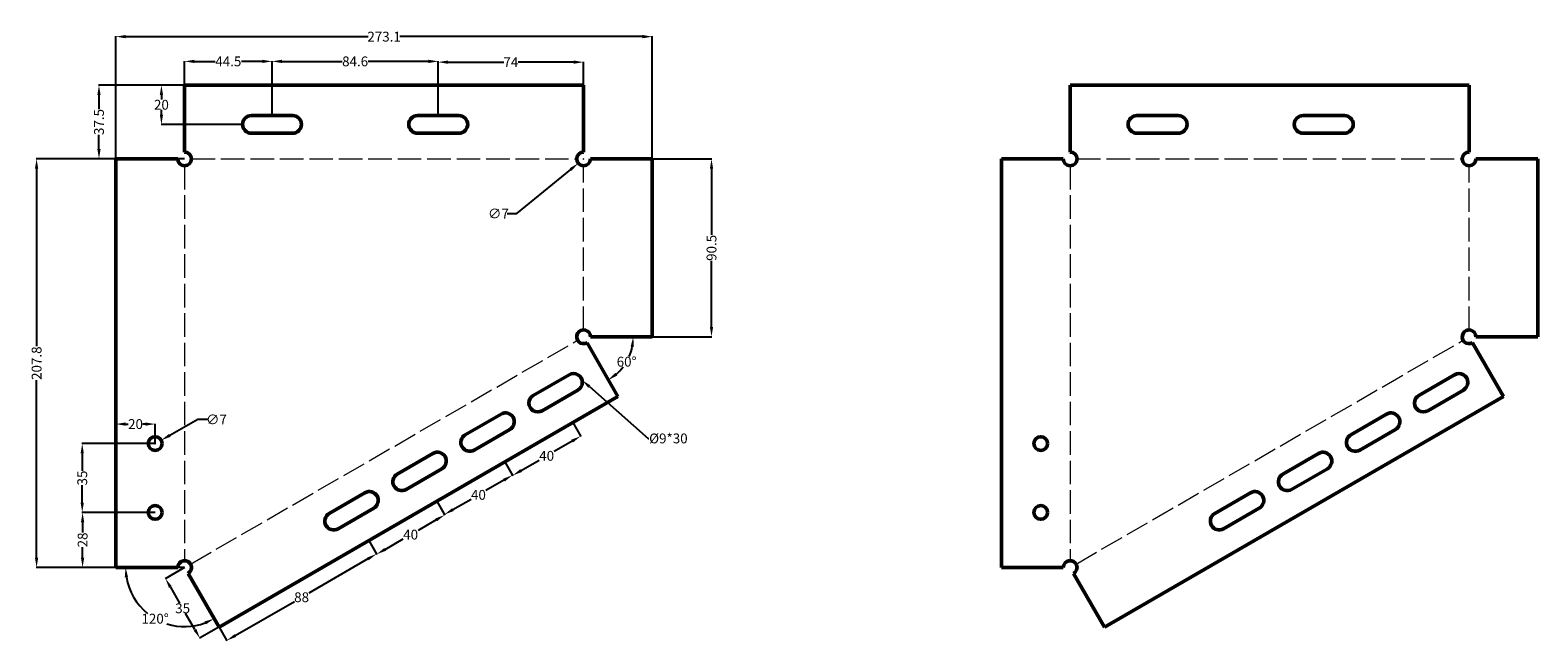
# Model space of a CAD drawing. Units: millimetres. Extents: x 105 to 872, y 91 to 402.
import ezdxf
from ezdxf import colors
from ezdxf.entities.mleader import LeaderData, LeaderLine
from ezdxf.math import Vec2, Vec3

# ---------------------------------------------------------------- set-up
doc = ezdxf.new("R2010")
doc.units = ezdxf.units.MM
doc.header["$MEASUREMENT"] = 0
doc.linetypes.add('ACAD_ISO02W100', pattern=[15, 12, -3])
for name, color, linetype, lineweight in [('M-BEND', 4, 'ACAD_ISO02W100', 18), ('M-DIMS', 3, 'Continuous', 25), ('M-OUTL', 7, 'Continuous', 50)]:
    doc.layers.add(name, color=color, linetype=linetype, lineweight=lineweight)
doc.styles.get("Standard").update_dxf_attribs({"font": 'arial.ttf'})
doc.dimstyles.get("Standard").update_dxf_attribs({"dimtxt": 5, "dimasz": 5, "dimexe": 0.18, "dimexo": 0.0625, "dimgap": 0.09, "dimtad": 0, "dimtih": 1, "dimtoh": 1, "dimdec": 1, "dimdsep": 46, "dimtxsty": 'Standard', "dimcen": 0.09, "dimadec": 0, "dimazin": 0, "dimtfac": 1, "dimtdec": 1, "dimtofl": 0, "dimtmove": 0, "dimatfit": 3, "dimfxl": 1, "dimtolj": 1, "dimtzin": 0, "dimarcsym": 0})

# ---------------------------------------------------------------- blocks, each defined once
blk = doc.blocks.new('*D1')
at = {"layer": 'Defpoints', "color": 0, "transparency": 16777216}
for p in [(386.49, 246.04), (386.49, 246.04), (421.49, 246.04), (405.87, 229.78), (403.99, 215.73)]:
    blk.add_point(p, dxfattribs=at)
at = {"layer": 'M-DIMS', "color": 0, "lineweight": -2, "transparency": 16777216}
for start, end in [(336.7044, 348.65824), (311.35025, 322.81457)]:
    blk.add_arc((386.49, 246.04), 25.3, start, end, dxfattribs=at)
at = {"layer": 'M-DIMS', "color": 0, "transparency": 16777216}
for points in [[(410.46, 241.14), (412.12, 240.98), (411.79, 246.04)], [(403.69, 226.37), (402.71, 227.72), (399.14, 224.13)]]:
    blk.add_solid(points, dxfattribs=at)
at = {"layer": 'M-DIMS', "color": 0, "transparency": 16777216, "insert": (408.4, 233.39), "char_height": 5, "attachment_point": 5}
blk.add_mtext('\\A1;60°', dxfattribs=at)
blk = doc.blocks.new('*D2')
at = {"layer": 'Defpoints', "color": 0, "transparency": 16777216}
for p in [(148.39, 128.74), (183.39, 128.74), (183.39, 128.74), (160.35, 109.41), (200.89, 98.43)]:
    blk.add_point(p, dxfattribs=at)
at = {"layer": 'M-DIMS', "color": 0, "lineweight": -2, "transparency": 16777216}
for start, end in [(189.53868, 231.09301), (252.54607, 290.46982)]:
    blk.add_arc((183.39, 128.74), 30.07, start, end, dxfattribs=at)
at = {"layer": 'M-DIMS', "color": 0, "transparency": 16777216}
for points in [[(152.9, 123.68), (154.56, 123.82), (153.32, 128.74)], [(193.55, 101.32), (194.26, 99.81), (198.42, 102.7)]]:
    blk.add_solid(points, dxfattribs=at)
at = {"layer": 'M-DIMS', "color": 0, "transparency": 16777216, "insert": (168.35, 102.7), "char_height": 5, "attachment_point": 5}
blk.add_mtext('\\A1;120°', dxfattribs=at)
blk = doc.blocks.new('*D3')
at = {"layer": 'Defpoints', "color": 0, "transparency": 16777216}
for p in [(183.39, 374.04), (171.57, 354.09), (212.89, 354.09)]:
    blk.add_point(p, dxfattribs=at)
at = {"layer": 'M-DIMS', "color": 0, "lineweight": -2, "transparency": 16777216}
for p, q in [((183.32, 374.04), (171.39, 374.04)), ((171.57, 369.04), (171.57, 366.7)), ((171.57, 359.09), (171.57, 361.42)), ((212.82, 354.09), (171.39, 354.09))]:
    blk.add_line(p, q, dxfattribs=at)
at = {"layer": 'M-DIMS', "color": 0, "transparency": 16777216}
for points in [[(170.74, 369.04), (172.41, 369.04), (171.57, 374.04)], [(170.74, 359.09), (172.41, 359.09), (171.57, 354.09)]]:
    blk.add_solid(points, dxfattribs=at)
at = {"layer": 'M-DIMS', "color": 0, "transparency": 16777216, "insert": (171.57, 364.06), "char_height": 5, "attachment_point": 5}
blk.add_mtext('\\A1;20', dxfattribs=at)
blk = doc.blocks.new('*D4')
at = {"layer": 'Defpoints', "color": 0, "transparency": 16777216}
for p in [(183.39, 374.04), (139.78, 336.54), (183.39, 336.54)]:
    blk.add_point(p, dxfattribs=at)
at = {"layer": 'M-DIMS', "color": 0, "lineweight": -2, "transparency": 16777216}
for p, q in [((183.32, 374.04), (139.6, 374.04)), ((139.78, 369.04), (139.78, 361.89)), ((139.78, 341.54), (139.78, 348.69)), ((183.32, 336.54), (139.6, 336.54))]:
    blk.add_line(p, q, dxfattribs=at)
at = {"layer": 'M-DIMS', "color": 0, "transparency": 16777216}
for points in [[(138.95, 369.04), (140.62, 369.04), (139.78, 374.04)], [(138.95, 341.54), (140.62, 341.54), (139.78, 336.54)]]:
    blk.add_solid(points, dxfattribs=at)
at = {"layer": 'M-DIMS', "color": 0, "transparency": 16777216, "insert": (139.78, 355.29), "char_height": 5, "attachment_point": 5, "rotation": 90}
blk.add_mtext('\\A1;37.5', dxfattribs=at)
blk = doc.blocks.new('*D5')
at = {"layer": 'Defpoints', "color": 0, "transparency": 16777216}
for p in [(421.49, 398.71), (148.39, 336.54), (421.49, 336.54)]:
    blk.add_point(p, dxfattribs=at)
at = {"layer": 'M-DIMS', "color": 0, "lineweight": -2, "transparency": 16777216}
for p, q in [((148.39, 336.6), (148.39, 398.89)), ((153.39, 398.71), (276.85, 398.71)), ((416.49, 398.71), (293.02, 398.71)), ((421.49, 336.6), (421.49, 398.89))]:
    blk.add_line(p, q, dxfattribs=at)
at = {"layer": 'M-DIMS', "color": 0, "transparency": 16777216}
for points in [[(153.39, 399.55), (153.39, 397.88), (148.39, 398.71)], [(416.49, 399.55), (416.49, 397.88), (421.49, 398.71)]]:
    blk.add_solid(points, dxfattribs=at)
at = {"layer": 'M-DIMS', "color": 0, "transparency": 16777216, "insert": (284.94, 398.71), "char_height": 5, "attachment_point": 5}
blk.add_mtext('\\A1;273.1', dxfattribs=at)
blk = doc.blocks.new('*D6')
at = {"layer": 'Defpoints', "color": 0, "transparency": 16777216}
for p in [(227.89, 386.13), (183.39, 374.04), (227.89, 358.59)]:
    blk.add_point(p, dxfattribs=at)
at = {"layer": 'M-DIMS', "color": 0, "lineweight": -2, "transparency": 16777216}
for p, q in [((183.39, 374.1), (183.39, 386.31)), ((188.39, 386.13), (198.93, 386.13)), ((222.89, 386.13), (212.34, 386.13)), ((227.89, 358.65), (227.89, 386.31))]:
    blk.add_line(p, q, dxfattribs=at)
at = {"layer": 'M-DIMS', "color": 0, "transparency": 16777216}
for points in [[(188.39, 386.96), (188.39, 385.29), (183.39, 386.13)], [(222.89, 386.96), (222.89, 385.29), (227.89, 386.13)]]:
    blk.add_solid(points, dxfattribs=at)
at = {"layer": 'M-DIMS', "color": 0, "transparency": 16777216, "insert": (205.64, 386.13), "char_height": 5, "attachment_point": 5}
blk.add_mtext('\\A1;44.5', dxfattribs=at)
blk = doc.blocks.new('*D7')
at = {"layer": 'Defpoints', "color": 0, "transparency": 16777216}
for p in [(312.49, 386.13), (227.89, 358.59), (312.49, 358.59)]:
    blk.add_point(p, dxfattribs=at)
at = {"layer": 'M-DIMS', "color": 0, "lineweight": -2, "transparency": 16777216}
for p, q in [((227.89, 358.65), (227.89, 386.31)), ((232.89, 386.13), (263.6, 386.13)), ((307.49, 386.13), (276.77, 386.13)), ((312.49, 358.65), (312.49, 386.31))]:
    blk.add_line(p, q, dxfattribs=at)
at = {"layer": 'M-DIMS', "color": 0, "transparency": 16777216}
for points in [[(232.89, 386.96), (232.89, 385.29), (227.89, 386.13)], [(307.49, 386.96), (307.49, 385.29), (312.49, 386.13)]]:
    blk.add_solid(points, dxfattribs=at)
at = {"layer": 'M-DIMS', "color": 0, "transparency": 16777216, "insert": (270.19, 386.13), "char_height": 5, "attachment_point": 5}
blk.add_mtext('\\A1;84.6', dxfattribs=at)
blk = doc.blocks.new('*D8')
at = {"layer": 'Defpoints', "color": 0, "transparency": 16777216}
for p in [(386.49, 385.75), (312.49, 358.59), (386.49, 358.59)]:
    blk.add_point(p, dxfattribs=at)
at = {"layer": 'M-DIMS', "color": 0, "lineweight": -2, "transparency": 16777216}
for p, q in [((312.49, 358.65), (312.49, 385.93)), ((317.49, 385.75), (345.84, 385.75)), ((381.49, 385.75), (353.13, 385.75)), ((386.49, 358.65), (386.49, 385.93))]:
    blk.add_line(p, q, dxfattribs=at)
at = {"layer": 'M-DIMS', "color": 0, "transparency": 16777216}
for points in [[(317.49, 386.58), (317.49, 384.91), (312.49, 385.75)], [(381.49, 386.58), (381.49, 384.91), (386.49, 385.75)]]:
    blk.add_solid(points, dxfattribs=at)
at = {"layer": 'M-DIMS', "color": 0, "transparency": 16777216, "insert": (349.49, 385.75), "char_height": 5, "attachment_point": 5}
blk.add_mtext('\\A1;74', dxfattribs=at)
blk = doc.blocks.new('*D9')
at = {"layer": 'Defpoints', "color": 0, "transparency": 16777216}
for p in [(131.43, 156.74), (168.39, 156.74), (148.39, 128.74)]:
    blk.add_point(p, dxfattribs=at)
at = {"layer": 'M-DIMS', "color": 0, "lineweight": -2, "transparency": 16777216}
for p, q in [((168.32, 156.74), (131.25, 156.74)), ((131.43, 151.74), (131.43, 146.46)), ((131.43, 133.74), (131.43, 139.02)), ((148.32, 128.74), (131.25, 128.74))]:
    blk.add_line(p, q, dxfattribs=at)
at = {"layer": 'M-DIMS', "color": 0, "transparency": 16777216}
for points in [[(130.6, 151.74), (132.27, 151.74), (131.43, 156.74)], [(130.6, 133.74), (132.27, 133.74), (131.43, 128.74)]]:
    blk.add_solid(points, dxfattribs=at)
at = {"layer": 'M-DIMS', "color": 0, "transparency": 16777216, "insert": (131.43, 142.74), "char_height": 5, "attachment_point": 5, "rotation": 90}
blk.add_mtext('\\A1;28', dxfattribs=at)
blk = doc.blocks.new('*D10')
at = {"layer": 'Defpoints', "color": 0, "transparency": 16777216}
for p in [(131.25, 191.74), (168.39, 191.74), (168.39, 156.74)]:
    blk.add_point(p, dxfattribs=at)
at = {"layer": 'M-DIMS', "color": 0, "lineweight": -2, "transparency": 16777216}
for p, q in [((168.32, 191.74), (131.07, 191.74)), ((131.25, 186.74), (131.25, 177.92)), ((131.25, 161.74), (131.25, 170.55)), ((168.32, 156.74), (131.07, 156.74))]:
    blk.add_line(p, q, dxfattribs=at)
at = {"layer": 'M-DIMS', "color": 0, "transparency": 16777216}
for points in [[(130.42, 186.74), (132.09, 186.74), (131.25, 191.74)], [(130.42, 161.74), (132.09, 161.74), (131.25, 156.74)]]:
    blk.add_solid(points, dxfattribs=at)
at = {"layer": 'M-DIMS', "color": 0, "transparency": 16777216, "insert": (131.25, 174.24), "char_height": 5, "attachment_point": 5, "rotation": 90}
blk.add_mtext('\\A1;35', dxfattribs=at)
blk = doc.blocks.new('*D11')
at = {"layer": 'Defpoints', "color": 0, "transparency": 16777216}
for p in [(148.39, 201.66), (148.39, 191.74), (168.39, 191.74)]:
    blk.add_point(p, dxfattribs=at)
at = {"layer": 'M-DIMS', "color": 0, "lineweight": -2, "transparency": 16777216}
for p, q in [((148.39, 191.8), (148.39, 201.84)), ((153.39, 201.66), (154.68, 201.66)), ((163.39, 201.66), (162.09, 201.66)), ((168.39, 191.8), (168.39, 201.84))]:
    blk.add_line(p, q, dxfattribs=at)
at = {"layer": 'M-DIMS', "color": 0, "transparency": 16777216}
for points in [[(153.39, 202.49), (153.39, 200.83), (148.39, 201.66)], [(163.39, 202.49), (163.39, 200.83), (168.39, 201.66)]]:
    blk.add_solid(points, dxfattribs=at)
at = {"layer": 'M-DIMS', "color": 0, "transparency": 16777216, "insert": (158.39, 201.66), "char_height": 5, "attachment_point": 5}
blk.add_mtext('\\A1;20', dxfattribs=at)
blk = doc.blocks.new('*D12')
at = {"layer": 'Defpoints', "color": 0, "transparency": 16777216}
for p in [(171.44, 193.45), (165.34, 190.02)]:
    blk.add_point(p, dxfattribs=at)
at = {"layer": 'M-DIMS', "color": 0, "lineweight": -2, "transparency": 16777216}
for p, q in [((190.14, 203.98), (175.79, 195.9)), ((195.14, 203.98), (190.14, 203.98)), ((168.3, 191.74), (168.48, 191.74)), ((168.39, 191.65), (168.39, 191.83))]:
    blk.add_line(p, q, dxfattribs=at)
at = {"layer": 'M-DIMS', "color": 0, "transparency": 16777216}
blk.add_solid([(175.38, 196.63), (176.2, 195.18), (171.44, 193.45)], dxfattribs=at)
at = {"layer": 'M-DIMS', "color": 0, "transparency": 16777216, "insert": (199.59, 203.98), "char_height": 5, "attachment_point": 5}
blk.add_mtext('\\A1;∅7', dxfattribs=at)
blk = doc.blocks.new('*D13')
at = {"layer": 'Defpoints', "color": 0, "transparency": 16777216}
for p in [(183.39, 336.54), (108.02, 128.74), (183.39, 128.74)]:
    blk.add_point(p, dxfattribs=at)
at = {"layer": 'M-DIMS', "color": 0, "lineweight": -2, "transparency": 16777216}
for p, q in [((183.32, 336.54), (107.84, 336.54)), ((108.02, 331.54), (108.02, 241.21)), ((108.02, 133.74), (108.02, 224.06)), ((183.32, 128.74), (107.84, 128.74))]:
    blk.add_line(p, q, dxfattribs=at)
at = {"layer": 'M-DIMS', "color": 0, "transparency": 16777216}
for points in [[(107.19, 331.54), (108.86, 331.54), (108.02, 336.54)], [(107.19, 133.74), (108.86, 133.74), (108.02, 128.74)]]:
    blk.add_solid(points, dxfattribs=at)
at = {"layer": 'M-DIMS', "color": 0, "transparency": 16777216, "insert": (108.02, 232.64), "char_height": 5, "attachment_point": 5, "rotation": 90}
blk.add_mtext('\\A1;207.8', dxfattribs=at)
blk = doc.blocks.new('*D14')
at = {"layer": 'Defpoints', "color": 0, "transparency": 16777216}
for p in [(389.19, 338.76), (383.78, 334.32)]:
    blk.add_point(p, dxfattribs=at)
at = {"layer": 'M-DIMS', "color": 0, "lineweight": -2, "transparency": 16777216}
for p, q in [((352.59, 308.71), (379.92, 331.14)), ((386.4, 336.54), (386.58, 336.54)), ((386.49, 336.45), (386.49, 336.63)), ((347.59, 308.71), (352.59, 308.71))]:
    blk.add_line(p, q, dxfattribs=at)
at = {"layer": 'M-DIMS', "color": 0, "transparency": 16777216}
blk.add_solid([(379.39, 331.79), (380.44, 330.5), (383.78, 334.32)], dxfattribs=at)
at = {"layer": 'M-DIMS', "color": 0, "transparency": 16777216, "insert": (343.14, 308.71), "char_height": 5, "attachment_point": 5}
blk.add_mtext('\\A1;∅7', dxfattribs=at)
blk = doc.blocks.new('*D15')
at = {"layer": 'Defpoints', "color": 0, "transparency": 16777216}
for p in [(421.49, 336.54), (421.49, 246.04), (451.62, 246.04)]:
    blk.add_point(p, dxfattribs=at)
at = {"layer": 'M-DIMS', "color": 0, "lineweight": -2, "transparency": 16777216}
for p, q in [((421.55, 336.54), (451.8, 336.54)), ((451.62, 331.54), (451.62, 297.89)), ((451.62, 251.04), (451.62, 284.68)), ((421.55, 246.04), (451.8, 246.04))]:
    blk.add_line(p, q, dxfattribs=at)
at = {"layer": 'M-DIMS', "color": 0, "transparency": 16777216}
for points in [[(450.79, 331.54), (452.45, 331.54), (451.62, 336.54)], [(450.79, 251.04), (452.45, 251.04), (451.62, 246.04)]]:
    blk.add_solid(points, dxfattribs=at)
at = {"layer": 'M-DIMS', "color": 0, "transparency": 16777216, "insert": (451.62, 291.29), "char_height": 5, "attachment_point": 5, "rotation": 90}
blk.add_mtext('\\A1;90.5', dxfattribs=at)
blk = doc.blocks.new('*D16')
at = {"layer": 'Defpoints', "color": 0, "transparency": 16777216}
for p in [(183.39, 128.74), (191.13, 92.79), (200.89, 98.43)]:
    blk.add_point(p, dxfattribs=at)
at = {"layer": 'M-DIMS', "color": 0, "lineweight": -2, "transparency": 16777216}
for p, q in [((183.33, 128.7), (173.47, 123.01)), ((176.13, 118.77), (180.85, 110.59)), ((188.63, 97.12), (183.91, 105.3)), ((200.84, 98.4), (190.98, 92.7))]:
    blk.add_line(p, q, dxfattribs=at)
at = {"layer": 'M-DIMS', "color": 0, "transparency": 16777216}
for points in [[(176.85, 119.19), (175.41, 118.35), (173.63, 123.1)], [(189.35, 97.54), (187.91, 96.71), (191.13, 92.79)]]:
    blk.add_solid(points, dxfattribs=at)
at = {"layer": 'M-DIMS', "color": 0, "transparency": 16777216, "insert": (182.38, 107.95), "char_height": 5, "attachment_point": 5}
blk.add_mtext('\\A1;35', dxfattribs=at)
blk = doc.blocks.new('*D17')
at = {"layer": 'Defpoints', "color": 0, "transparency": 16777216}
for p in [(277.09, 142.44), (281.04, 135.6), (200.89, 98.43)]:
    blk.add_point(p, dxfattribs=at)
at = {"layer": 'M-DIMS', "color": 0, "lineweight": -2, "transparency": 16777216}
for p, q in [((277.12, 142.39), (281.13, 135.45)), ((276.71, 133.1), (246.62, 115.72)), ((209.17, 94.09), (239.26, 111.47)), ((200.92, 98.37), (204.93, 91.43))]:
    blk.add_line(p, q, dxfattribs=at)
at = {"layer": 'M-DIMS', "color": 0, "transparency": 16777216}
for points in [[(276.3, 133.82), (277.13, 132.38), (281.04, 135.6)], [(208.75, 94.81), (209.59, 93.37), (204.84, 91.59)]]:
    blk.add_solid(points, dxfattribs=at)
at = {"layer": 'M-DIMS', "color": 0, "transparency": 16777216, "insert": (242.94, 113.6), "char_height": 5, "attachment_point": 5}
blk.add_mtext('\\A1;88', dxfattribs=at)
blk = doc.blocks.new('*D18')
at = {"layer": 'Defpoints', "color": 0, "transparency": 16777216}
for p in [(311.73, 162.44), (315.77, 155.45), (277.09, 142.44)]:
    blk.add_point(p, dxfattribs=at)
at = {"layer": 'M-DIMS', "color": 0, "lineweight": -2, "transparency": 16777216}
for p, q in [((311.76, 162.39), (315.86, 155.3)), ((311.44, 152.95), (302.21, 147.62)), ((277.12, 142.39), (281.22, 135.29)), ((285.46, 137.95), (294.69, 143.27))]:
    blk.add_line(p, q, dxfattribs=at)
at = {"layer": 'M-DIMS', "color": 0, "transparency": 16777216}
for points in [[(311.02, 153.67), (311.86, 152.23), (315.77, 155.45)], [(285.05, 138.67), (285.88, 137.22), (281.13, 135.45)]]:
    blk.add_solid(points, dxfattribs=at)
at = {"layer": 'M-DIMS', "color": 0, "transparency": 16777216, "insert": (298.45, 145.45), "char_height": 5, "attachment_point": 5}
blk.add_mtext('\\A1;40', dxfattribs=at)
blk = doc.blocks.new('*D19')
at = {"layer": 'Defpoints', "color": 0, "transparency": 16777216}
for p in [(346.37, 182.45), (350.28, 175.67), (311.73, 162.44)]:
    blk.add_point(p, dxfattribs=at)
at = {"layer": 'M-DIMS', "color": 0, "lineweight": -2, "transparency": 16777216}
for p, q in [((346.4, 182.4), (350.37, 175.52)), ((345.95, 173.17), (336.73, 167.84)), ((311.76, 162.39), (315.74, 155.51)), ((319.98, 158.17), (329.2, 163.5))]:
    blk.add_line(p, q, dxfattribs=at)
at = {"layer": 'M-DIMS', "color": 0, "transparency": 16777216}
for points in [[(345.54, 173.89), (346.37, 172.45), (350.28, 175.67)], [(319.56, 158.89), (320.39, 157.45), (315.65, 155.67)]]:
    blk.add_solid(points, dxfattribs=at)
at = {"layer": 'M-DIMS', "color": 0, "transparency": 16777216, "insert": (332.96, 165.67), "char_height": 5, "attachment_point": 5}
blk.add_mtext('\\A1;40', dxfattribs=at)
blk = doc.blocks.new('*D20')
at = {"layer": 'Defpoints', "color": 0, "transparency": 16777216}
for p in [(381.01, 202.45), (385.01, 195.52), (346.37, 182.45)]:
    blk.add_point(p, dxfattribs=at)
at = {"layer": 'M-DIMS', "color": 0, "lineweight": -2, "transparency": 16777216}
for p, q in [((381.04, 202.4), (385.1, 195.37)), ((380.68, 193.02), (371.46, 187.69)), ((346.4, 182.4), (350.46, 175.36)), ((354.7, 178.02), (363.93, 183.35))]:
    blk.add_line(p, q, dxfattribs=at)
at = {"layer": 'M-DIMS', "color": 0, "transparency": 16777216}
for points in [[(380.27, 193.74), (381.1, 192.3), (385.01, 195.52)], [(354.29, 178.74), (355.12, 177.3), (350.37, 175.52)]]:
    blk.add_solid(points, dxfattribs=at)
at = {"layer": 'M-DIMS', "color": 0, "transparency": 16777216, "insert": (367.69, 185.52), "char_height": 5, "attachment_point": 5}
blk.add_mtext('\\A1;40', dxfattribs=at)

msp = doc.modelspace()

# ---------------------------------------------------------------- linework, layer by layer
at = {"layer": 'M-BEND'}
for p, q in [((183.39, 333.04), (183.39, 132.24)), ((186.89, 336.54), (382.99, 336.54)), ((386.49, 249.54), (386.49, 333.04)), ((634.22, 333.04), (634.22, 132.24)), ((637.72, 336.54), (833.82, 336.54)), ((837.32, 249.54), (837.32, 333.04)), ((186.42, 130.49), (383.45, 244.29)), ((637.25, 130.49), (834.29, 244.29))]:
    msp.add_line(p, q, dxfattribs=at)
at = {"layer": 'M-OUTL'}
for p, q in [((183.39, 340.04), (183.39, 374.04)), ((386.49, 374.04), (183.39, 374.04)), ((386.49, 340.04), (386.49, 374.04)), ((634.22, 340.04), (634.22, 374.04)), ((837.32, 374.04), (634.22, 374.04)), ((837.32, 340.04), (837.32, 374.04)), ((148.39, 128.74), (148.39, 336.54)), ((148.39, 336.54), (179.89, 336.54)), ((389.99, 336.54), (421.49, 336.54)), ((421.49, 336.54), (421.49, 246.04)), ((599.22, 128.74), (599.22, 336.54)), ((599.22, 336.54), (630.72, 336.54)), ((840.82, 336.54), (872.32, 336.54)), ((872.32, 336.54), (872.32, 246.04)), ((421.49, 246.04), (389.99, 246.04)), ((872.32, 246.04), (840.82, 246.04)), ((388.24, 243.01), (403.99, 215.73)), ((839.07, 243.01), (854.82, 215.73)), ((200.89, 98.43), (403.99, 215.73)), ((651.72, 98.43), (854.82, 215.73)), ((148.39, 128.74), (179.89, 128.74)), ((185.14, 125.71), (200.89, 98.43)), ((599.22, 128.74), (630.72, 128.74)), ((635.97, 125.71), (651.72, 98.43))]:
    msp.add_line(p, q, dxfattribs=at)
for points in [[(238.39, 358.59, -1), (238.39, 349.59), (217.39, 349.59, -1), (217.39, 358.59)], [(322.99, 358.59, -1), (322.99, 349.59), (301.99, 349.59, -1), (301.99, 358.59)], [(689.22, 358.59, -1), (689.22, 349.59), (668.22, 349.59, -1), (668.22, 358.59)], [(773.82, 358.59, -1), (773.82, 349.59), (752.82, 349.59, -1), (752.82, 358.59)], [(379.1, 226.76, -1), (383.6, 218.96), (365.41, 208.46, -1), (360.91, 216.26)], [(829.93, 226.76, -1), (834.43, 218.96), (816.24, 208.46, -1), (811.74, 216.26)], [(344.46, 206.75, -1), (348.96, 198.96), (330.77, 188.46, -1), (326.27, 196.25)], [(795.29, 206.75, -1), (799.79, 198.96), (781.61, 188.46, -1), (777.11, 196.25)], [(309.82, 186.75, -1), (314.32, 178.95), (296.14, 168.45, -1), (291.64, 176.25)], [(760.65, 186.75, -1), (765.15, 178.95), (746.97, 168.45, -1), (742.47, 176.25)], [(275.18, 166.74, -1), (279.68, 158.95), (261.5, 148.45, -1), (257, 156.24)], [(726.02, 166.74, -1), (730.52, 158.95), (712.33, 148.45, -1), (707.83, 156.24)]]:
    msp.add_lwpolyline(points, format="xyb", close=True, dxfattribs=at)
for centre in [(168.39, 191.74), (619.22, 191.74), (168.39, 156.74), (619.22, 156.74)]:
    msp.add_circle(centre, 3.5, dxfattribs=at)
for centre, start, end in [((183.39, 336.54), 180, 90), ((386.49, 336.54), 90, 0), ((634.22, 336.54), 180, 90), ((837.32, 336.54), 90, 0), ((386.49, 246.04), 0, 300.0085), ((837.32, 246.04), 0, 300.0085), ((183.39, 128.74), 300.0085, 180), ((634.22, 128.74), 300.0085, 180)]:
    msp.add_arc(centre, 3.5, start, end, dxfattribs=at)

# ---------------------------------------------------------------- dimensions: what is measured, and where the dimension line sits
at = {"layer": 'M-DIMS', "transparency": 33554610}
for base, p1, p2, picture, middle in [((421.49, 398.71), (148.39, 336.54), (421.49, 336.54), '*D5', (284.94, 398.71)), ((227.89, 386.13), (183.39, 374.04), (227.89, 358.59), '*D6', (205.64, 386.13)), ((312.49, 386.13), (227.89, 358.59), (312.49, 358.59), '*D7', (270.19, 386.13)), ((386.49, 385.75), (312.49, 358.59), (386.49, 358.59), '*D8', (349.49, 385.75)), ((148.39, 201.66), (168.39, 191.74), (148.39, 191.74), '*D11', (158.39, 201.66))]:
    dim = msp.add_linear_dim(base=base, p1=p1, p2=p2, dimstyle='Standard', override={"dimclrd": 0, "dimclre": 0, "dimclrt": 0}, dxfattribs=at)
    dim.commit()
    dim.dimension.update_dxf_attribs({"geometry": picture, "text_midpoint": middle})
for base, p1, p2, picture, middle in [((139.78, 336.54), (183.39, 374.04), (183.39, 336.54), '*D4', (139.78, 355.29)), ((108.02, 128.74), (183.39, 336.54), (183.39, 128.74), '*D13', (108.02, 232.64)), ((451.62, 246.04), (421.49, 336.54), (421.49, 246.04), '*D15', (451.62, 291.29)), ((131.25, 191.74), (168.39, 156.74), (168.39, 191.74), '*D10', (131.25, 174.24)), ((131.43, 156.74), (148.39, 128.74), (168.39, 156.74), '*D9', (131.43, 142.74))]:
    dim = msp.add_linear_dim(base=base, p1=p1, p2=p2, angle=90, dimstyle='Standard', override={"dimclrd": 0, "dimclre": 0, "dimclrt": 0}, dxfattribs=at)
    dim.commit()
    dim.dimension.update_dxf_attribs({"geometry": picture, "text_midpoint": middle, "text_rotation": 90})
dim = msp.add_linear_dim(base=(171.57215553, 354.08621907), p1=(183.38542314, 374.03621907), p2=(212.88542314, 354.08621907), angle=90, dimstyle='Standard', override={"dimclrd": 0, "dimclre": 0, "dimclrt": 0}, dxfattribs=at)
dim.commit()
dim.dimension.update_dxf_attribs({"geometry": '*D3', "text_midpoint": (171.57215553, 364.06121907)})
for p1, p2, picture, middle in [((389.19, 338.76), (383.78, 334.32), '*D14', (343.14, 308.71)), ((165.34, 190.02), (171.44, 193.45), '*D12', (199.59, 203.98))]:
    dim = msp.add_diameter_dim_2p(p1=p1, p2=p2, dimstyle='Standard', override={"dimclrd": 0, "dimclre": 0, "dimclrt": 0}, dxfattribs=at)
    dim.commit()
    dim.dimension.update_dxf_attribs({"geometry": picture, "text_midpoint": middle, "dimtype": 163})
for base, line1, line2, picture, middle in [((405.87, 229.78), ((421.49, 246.04), (386.49, 246.04)), ((386.49, 246.04), (403.99, 215.73)), '*D1', (408.4, 233.39)), ((160.35, 109.41), ((183.39, 128.74), (200.89, 98.43)), ((148.39, 128.74), (183.39, 128.74)), '*D2', (168.35, 102.7))]:
    dim = msp.add_angular_dim_2l(base=base, line1=line1, line2=line2, dimstyle='Standard', override={"dimclrd": 0, "dimclre": 0, "dimclrt": 0}, dxfattribs=at)
    dim.commit()
    dim.dimension.update_dxf_attribs({"geometry": picture, "text_midpoint": middle})
for p1, p2, distance, picture, middle in [((346.37, 182.45), (381.01, 202.45), -8.01, '*D20', (367.69, 185.52)), ((311.73, 162.44), (346.37, 182.45), -7.83, '*D19', (332.96, 165.67)), ((277.09, 142.44), (311.73, 162.44), -8.08, '*D18', (298.45, 145.45)), ((200.89, 98.43), (277.09, 142.44), -7.9, '*D17', (242.94, 113.6)), ((183.39, 128.74), (200.89, 98.43), -11.27, '*D16', (182.38, 107.95))]:
    dim = msp.add_aligned_dim(p1=p1, p2=p2, distance=distance, dimstyle='Standard', override={"dimclrd": 0, "dimclre": 0, "dimclrt": 0}, dxfattribs=at)
    dim.commit()
    dim.dimension.update_dxf_attribs({"geometry": picture, "text_midpoint": middle})

# ---------------------------------------------------------------- leaders
ml = msp.add_multileader_mtext('Standard', dxfattribs=at)
ml.set_content('%%C9*30', color=256)
ml.set_leader_properties()
ml.build(insert=Vec2(0, 0))
ml.multileader.update_dxf_attribs({"dogleg_length": 0.36, "arrow_head_size": 5})
ctx = ml.context
ctx.base_point, ctx.char_height, ctx.arrow_head_size, ctx.landing_gap_size, ctx.plane_origin = Vec3(419.78, 194.26), 5, 5, 0.09, Vec3(386.67, 224.29)
notes = []
notes.append((ctx, [(0, (1, 1, 0), (419.42, 194.26), (1, 0), 0.36, [(0, [(385.7, 224.02)], 0, [])])]))
ctx.mtext.insert, ctx.mtext.flow_direction = Vec3(419.87, 196.86), 5
for ctx, leaders in notes:
    for number, flags, end, landing, length, lines in leaders:
        leader = LeaderData()
        leader.index, (leader.has_last_leader_line, leader.has_dogleg_vector, leader.attachment_direction) = number, flags
        leader.last_leader_point, leader.dogleg_vector, leader.dogleg_length = Vec3(end), Vec3(landing), length
        for number, points, colour, breaks in lines:
            line = LeaderLine()
            line.index, line.vertices, line.color, line.breaks = number, Vec3.list(points), colors.encode_raw_color(colour), breaks
            leader.lines.append(line)
        ctx.leaders.append(leader)

doc.saveas('drawing.dxf')
